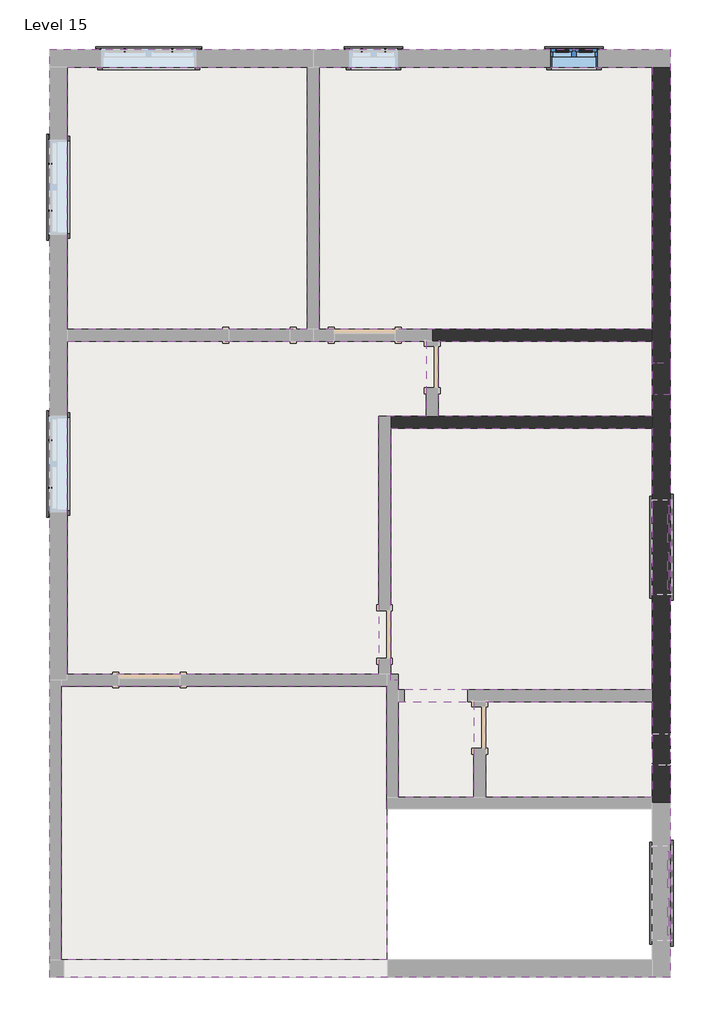
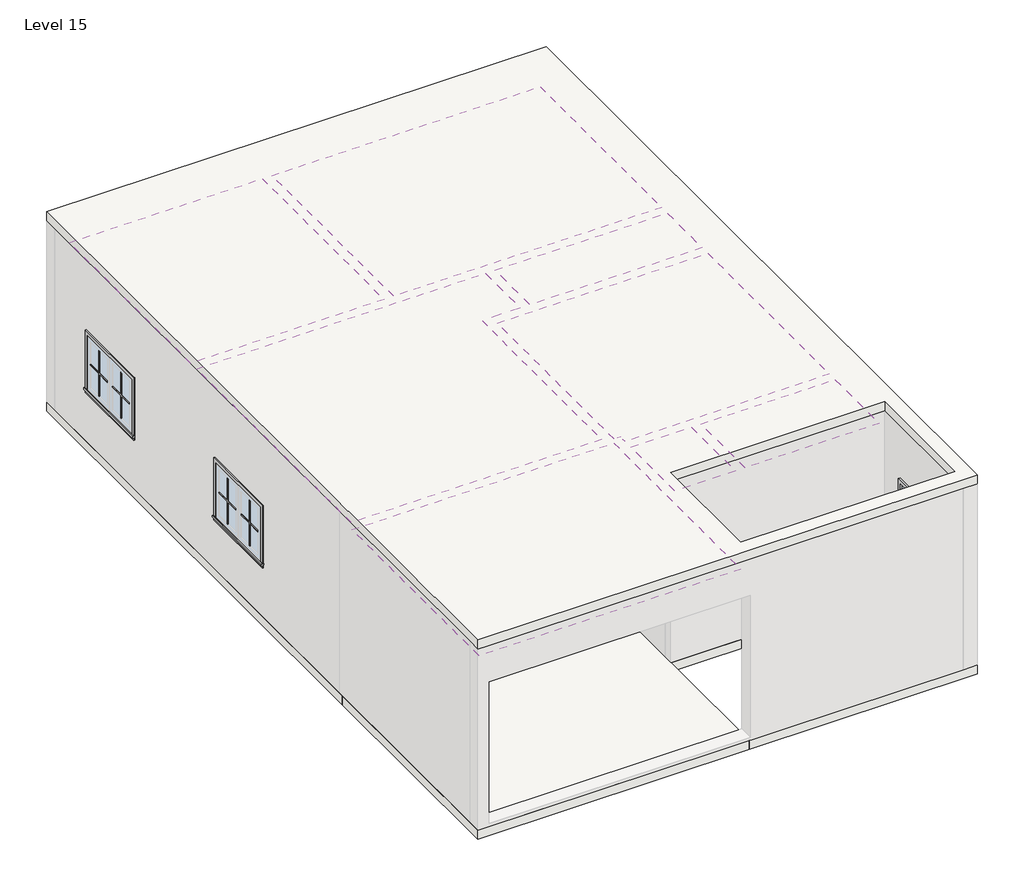
# One storey, part 2 of 2: 44 proxies, 8 coverings, 3 slabs, 3 walls, 3 windows.
"""IFC4 building model written with IfcOpenShell, lengths in millimetres."""

from ifc_helpers import new_model, si_unit, frame, origin, place, context, project, spatial, polyline, outline, extrude, faceted_brep, transform, mapped, element, save
from components import muntin_pattern_2x2_muntin_pattern_2x2_2357e71d, muntin_pattern_2x2_muntin_pattern_2x2_302d8f29, muntin_pattern_2x2_muntin_pattern_2x2_53152e2c, muntin_pattern_2x2_muntin_pattern_2x2_e8f3e573, trim_window_exterior_flat_with_sill_c4e67c73, trim_window_exterior_flat_with_sill_a665a915, trim_window_interior_flat_picture_frame_cf1733af, trim_window_interior_flat_picture_frame_d485c387, fixed_2_415b3208, window_casement_double_3_c417fced

model = new_model("IFC4")

# Units and contexts
model_context = context("Model", 3, world=origin())
ifc_project = project(units=[si_unit("LENGTHUNIT", "METRE", prefix="MILLI")], contexts=[model_context])

# Site, building, storey
site = spatial("IfcSite", under=ifc_project)
building = spatial("IfcBuilding", under=site)
storey = spatial("IfcBuildingStorey", under=building, Name="Level 15", Elevation=6400.8)

# Proxies
placement = place(None, origin())
muntin_pattern_2x2_muntin_pattern_2x2_shape = muntin_pattern_2x2_muntin_pattern_2x2_2357e71d(model_context)
element("IfcBuildingElementProxy", 1, Name="Muntin Pattern_2x2 : Muntin Pattern_2x2", ObjectType="Muntin Pattern_2x2 : Muntin Pattern_2x2", at=placement, inside=storey, context=model_context, shape_type="MappedRepresentation", body=[
    mapped(muntin_pattern_2x2_muntin_pattern_2x2_shape, transform((-4942.3279463, 5897.3080275, 7385.05), x_axis=(1.0, 0.0, 0.0), y_axis=(0.0, 1.0, 0.0), z_axis=(0.0, 0.0, 1.0))),
])
element("IfcBuildingElementProxy", 2, Name="Muntin Pattern_2x2 : Muntin Pattern_2x2", ObjectType="Muntin Pattern_2x2 : Muntin Pattern_2x2", at=placement, inside=storey, context=model_context, shape_type="MappedRepresentation", body=[
    mapped(muntin_pattern_2x2_muntin_pattern_2x2_shape, transform((-5899.5904463, 3838.3205275, 7385.05), x_axis=(0.0, 1.0, 0.0), y_axis=(-1.0, 0.0, 0.0), z_axis=(0.0, 0.0, 1.0))),
])
element("IfcBuildingElementProxy", 3, Name="Muntin Pattern_2x2 : Muntin Pattern_2x2", ObjectType="Muntin Pattern_2x2 : Muntin Pattern_2x2", at=placement, inside=storey, context=model_context, shape_type="MappedRepresentation", body=[
    mapped(muntin_pattern_2x2_muntin_pattern_2x2_shape, transform((-5899.5904463, 293.4330275, 7385.05), x_axis=(0.0, 1.0, 0.0), y_axis=(-1.0, 0.0, 0.0), z_axis=(0.0, 0.0, 1.0))),
])
element("IfcBuildingElementProxy", 4, Name="Muntin Pattern_2x2 : Muntin Pattern_2x2", ObjectType="Muntin Pattern_2x2 : Muntin Pattern_2x2", at=placement, inside=storey, context=model_context, shape_type="MappedRepresentation", body=[
    mapped(muntin_pattern_2x2_muntin_pattern_2x2_shape, transform((2031.5595537, -166.9419725, 7689.85), x_axis=(0.0, -1.0, 0.0), y_axis=(1.0, 0.0, 0.0), z_axis=(0.0, 0.0, 1.0))),
])
element("IfcBuildingElementProxy", 5, Name="Muntin Pattern_2x2 : Muntin Pattern_2x2", ObjectType="Muntin Pattern_2x2 : Muntin Pattern_2x2", at=placement, inside=storey, context=model_context, shape_type="MappedRepresentation", body=[
    mapped(muntin_pattern_2x2_muntin_pattern_2x2_shape, transform((2031.5595537, -4599.2419725, 7689.85), x_axis=(0.0, -1.0, 0.0), y_axis=(1.0, 0.0, 0.0), z_axis=(0.0, 0.0, 1.0))),
])
element("IfcBuildingElementProxy", 6, Name="Muntin Pattern_2x2 : Muntin Pattern_2x2", ObjectType="Muntin Pattern_2x2 : Muntin Pattern_2x2", at=placement, inside=storey, context=model_context, shape_type="MappedRepresentation", body=[
    mapped(muntin_pattern_2x2_muntin_pattern_2x2_shape, transform((-4942.3279463, 5897.3080275, 7385.05), x_axis=(1.0, 0.0, 0.0), y_axis=(0.0, 1.0, 0.0), z_axis=(0.0, 0.0, 1.0))),
])
element("IfcBuildingElementProxy", 7, Name="Muntin Pattern_2x2 : Muntin Pattern_2x2", ObjectType="Muntin Pattern_2x2 : Muntin Pattern_2x2", at=placement, inside=storey, context=model_context, shape_type="MappedRepresentation", body=[
    mapped(muntin_pattern_2x2_muntin_pattern_2x2_shape, transform((2031.5595537, -4599.2419725, 7689.85), x_axis=(0.0, -1.0, 0.0), y_axis=(1.0, 0.0, 0.0), z_axis=(0.0, 0.0, 1.0))),
])
muntin_pattern_2x2_muntin_pattern_2x2_2_shape = muntin_pattern_2x2_muntin_pattern_2x2_302d8f29(model_context)
element("IfcBuildingElementProxy", 8, Name="Muntin Pattern_2x2 : Muntin Pattern_2x2", ObjectType="Muntin Pattern_2x2 : Muntin Pattern_2x2", at=placement, inside=storey, context=model_context, shape_type="MappedRepresentation", body=[
    mapped(muntin_pattern_2x2_muntin_pattern_2x2_2_shape, transform((-4335.9029463, 5897.3080275, 7385.05), x_axis=(-1.0, 0.0, 0.0), y_axis=(0.0, -1.0, 0.0), z_axis=(0.0, 0.0, 1.0))),
])
element("IfcBuildingElementProxy", 9, Name="Muntin Pattern_2x2 : Muntin Pattern_2x2", ObjectType="Muntin Pattern_2x2 : Muntin Pattern_2x2", at=placement, inside=storey, context=model_context, shape_type="MappedRepresentation", body=[
    mapped(muntin_pattern_2x2_muntin_pattern_2x2_2_shape, transform((-5899.5904463, 4444.7455275, 7385.05), x_axis=(0.0, -1.0, 0.0), y_axis=(1.0, 0.0, 0.0), z_axis=(0.0, 0.0, 1.0))),
])
element("IfcBuildingElementProxy", 10, Name="Muntin Pattern_2x2 : Muntin Pattern_2x2", ObjectType="Muntin Pattern_2x2 : Muntin Pattern_2x2", at=placement, inside=storey, context=model_context, shape_type="MappedRepresentation", body=[
    mapped(muntin_pattern_2x2_muntin_pattern_2x2_2_shape, transform((-5899.5904463, 899.8580275, 7385.05), x_axis=(0.0, -1.0, 0.0), y_axis=(1.0, 0.0, 0.0), z_axis=(0.0, 0.0, 1.0))),
])
element("IfcBuildingElementProxy", 11, Name="Muntin Pattern_2x2 : Muntin Pattern_2x2", ObjectType="Muntin Pattern_2x2 : Muntin Pattern_2x2", at=placement, inside=storey, context=model_context, shape_type="MappedRepresentation", body=[
    mapped(muntin_pattern_2x2_muntin_pattern_2x2_2_shape, transform((2031.5595537, -773.3669725, 7689.85), x_axis=(0.0, 1.0, 0.0), y_axis=(-1.0, 0.0, 0.0), z_axis=(0.0, 0.0, 1.0))),
])
element("IfcBuildingElementProxy", 12, Name="Muntin Pattern_2x2 : Muntin Pattern_2x2", ObjectType="Muntin Pattern_2x2 : Muntin Pattern_2x2", at=placement, inside=storey, context=model_context, shape_type="MappedRepresentation", body=[
    mapped(muntin_pattern_2x2_muntin_pattern_2x2_2_shape, transform((2031.5595537, -5205.6669725, 7689.85), x_axis=(0.0, 1.0, 0.0), y_axis=(-1.0, 0.0, 0.0), z_axis=(0.0, 0.0, 1.0))),
])
element("IfcBuildingElementProxy", 13, Name="Muntin Pattern_2x2 : Muntin Pattern_2x2", ObjectType="Muntin Pattern_2x2 : Muntin Pattern_2x2", at=placement, inside=storey, context=model_context, shape_type="MappedRepresentation", body=[
    mapped(muntin_pattern_2x2_muntin_pattern_2x2_2_shape, transform((-4335.9029463, 5897.3080275, 7385.05), x_axis=(-1.0, 0.0, 0.0), y_axis=(0.0, -1.0, 0.0), z_axis=(0.0, 0.0, 1.0))),
])
element("IfcBuildingElementProxy", 14, Name="Muntin Pattern_2x2 : Muntin Pattern_2x2", ObjectType="Muntin Pattern_2x2 : Muntin Pattern_2x2", at=placement, inside=storey, context=model_context, shape_type="MappedRepresentation", body=[
    mapped(muntin_pattern_2x2_muntin_pattern_2x2_2_shape, transform((2031.5595537, -5205.6669725, 7689.85), x_axis=(0.0, 1.0, 0.0), y_axis=(-1.0, 0.0, 0.0), z_axis=(0.0, 0.0, 1.0))),
])
muntin_pattern_2x2_muntin_pattern_2x2_3_shape = muntin_pattern_2x2_muntin_pattern_2x2_53152e2c(model_context)
element("IfcBuildingElementProxy", 15, Name="Muntin Pattern_2x2 : Muntin Pattern_2x2", ObjectType="Muntin Pattern_2x2 : Muntin Pattern_2x2", at=placement, inside=storey, context=model_context, shape_type="MappedRepresentation", body=[
    mapped(muntin_pattern_2x2_muntin_pattern_2x2_3_shape, transform((-1907.0279463, 5897.3080275, 7385.05), x_axis=(1.0, 0.0, 0.0), y_axis=(0.0, 1.0, 0.0), z_axis=(0.0, 0.0, 1.0))),
])
element("IfcBuildingElementProxy", 16, Name="Muntin Pattern_2x2 : Muntin Pattern_2x2", ObjectType="Muntin Pattern_2x2 : Muntin Pattern_2x2", at=placement, inside=storey, context=model_context, shape_type="MappedRepresentation", body=[
    mapped(muntin_pattern_2x2_muntin_pattern_2x2_3_shape, transform((658.3720537, 5897.3080275, 7385.05), x_axis=(1.0, 0.0, 0.0), y_axis=(0.0, 1.0, 0.0), z_axis=(0.0, 0.0, 1.0))),
])
element("IfcBuildingElementProxy", 17, Name="Muntin Pattern_2x2 : Muntin Pattern_2x2", ObjectType="Muntin Pattern_2x2 : Muntin Pattern_2x2", at=placement, inside=storey, context=model_context, shape_type="MappedRepresentation", body=[
    mapped(muntin_pattern_2x2_muntin_pattern_2x2_3_shape, transform((-1907.0279463, 5897.3080275, 7385.05), x_axis=(1.0, 0.0, 0.0), y_axis=(0.0, 1.0, 0.0), z_axis=(0.0, 0.0, 1.0))),
])
element("IfcBuildingElementProxy", 18, Name="Muntin Pattern_2x2 : Muntin Pattern_2x2", ObjectType="Muntin Pattern_2x2 : Muntin Pattern_2x2", at=placement, inside=storey, context=model_context, shape_type="MappedRepresentation", body=[
    mapped(muntin_pattern_2x2_muntin_pattern_2x2_3_shape, transform((658.3720537, 5897.3080275, 7385.05), x_axis=(1.0, 0.0, 0.0), y_axis=(0.0, 1.0, 0.0), z_axis=(0.0, 0.0, 1.0))),
])
muntin_pattern_2x2_muntin_pattern_2x2_4_shape = muntin_pattern_2x2_muntin_pattern_2x2_e8f3e573(model_context)
element("IfcBuildingElementProxy", 19, Name="Muntin Pattern_2x2 : Muntin Pattern_2x2", ObjectType="Muntin Pattern_2x2 : Muntin Pattern_2x2", at=placement, inside=storey, context=model_context, shape_type="MappedRepresentation", body=[
    mapped(muntin_pattern_2x2_muntin_pattern_2x2_4_shape, transform((-1605.4029463, 5897.3080275, 7385.05), x_axis=(-1.0, 0.0, 0.0), y_axis=(0.0, -1.0, 0.0), z_axis=(0.0, 0.0, 1.0))),
])
element("IfcBuildingElementProxy", 20, Name="Muntin Pattern_2x2 : Muntin Pattern_2x2", ObjectType="Muntin Pattern_2x2 : Muntin Pattern_2x2", at=placement, inside=storey, context=model_context, shape_type="MappedRepresentation", body=[
    mapped(muntin_pattern_2x2_muntin_pattern_2x2_4_shape, transform((959.9970537, 5897.3080275, 7385.05), x_axis=(-1.0, 0.0, 0.0), y_axis=(0.0, -1.0, 0.0), z_axis=(0.0, 0.0, 1.0))),
])
element("IfcBuildingElementProxy", 21, Name="Muntin Pattern_2x2 : Muntin Pattern_2x2", ObjectType="Muntin Pattern_2x2 : Muntin Pattern_2x2", at=placement, inside=storey, context=model_context, shape_type="MappedRepresentation", body=[
    mapped(muntin_pattern_2x2_muntin_pattern_2x2_4_shape, transform((-1605.4029463, 5897.3080275, 7385.05), x_axis=(-1.0, 0.0, 0.0), y_axis=(0.0, -1.0, 0.0), z_axis=(0.0, 0.0, 1.0))),
])
element("IfcBuildingElementProxy", 22, Name="Muntin Pattern_2x2 : Muntin Pattern_2x2", ObjectType="Muntin Pattern_2x2 : Muntin Pattern_2x2", at=placement, inside=storey, context=model_context, shape_type="MappedRepresentation", body=[
    mapped(muntin_pattern_2x2_muntin_pattern_2x2_4_shape, transform((959.9970537, 5897.3080275, 7385.05), x_axis=(-1.0, 0.0, 0.0), y_axis=(0.0, -1.0, 0.0), z_axis=(0.0, 0.0, 1.0))),
])
trim_window_exterior_flat_with_sill_shape = trim_window_exterior_flat_with_sill_c4e67c73(model_context)
element("IfcBuildingElementProxy", 23, Name="Trim-Window-Exterior-Flat : with Sill", ObjectType="Trim-Window-Exterior-Flat : with Sill", at=placement, inside=storey, context=model_context, shape_type="MappedRepresentation", body=[
    mapped(trim_window_exterior_flat_with_sill_shape, transform((-4639.1154463, 5906.8330275, 8229.6), x_axis=(-1.0, 0.0, 0.0), y_axis=(0.0, 0.0, 1.0), z_axis=(0.0, 1.0, 0.0))),
])
element("IfcBuildingElementProxy", 24, Name="Trim-Window-Exterior-Flat : with Sill", ObjectType="Trim-Window-Exterior-Flat : with Sill", at=placement, inside=storey, context=model_context, shape_type="MappedRepresentation", body=[
    mapped(trim_window_exterior_flat_with_sill_shape, transform((-5909.1154463, 4141.5330275, 8229.6), x_axis=(0.0, -1.0, 0.0), y_axis=(0.0, 0.0, 1.0), z_axis=(-1.0, 0.0, 0.0))),
])
element("IfcBuildingElementProxy", 25, Name="Trim-Window-Exterior-Flat : with Sill", ObjectType="Trim-Window-Exterior-Flat : with Sill", at=placement, inside=storey, context=model_context, shape_type="MappedRepresentation", body=[
    mapped(trim_window_exterior_flat_with_sill_shape, transform((-5909.1154463, 596.6455275, 8229.6), x_axis=(0.0, -1.0, 0.0), y_axis=(0.0, 0.0, 1.0), z_axis=(-1.0, 0.0, 0.0))),
])
element("IfcBuildingElementProxy", 26, Name="Trim-Window-Exterior-Flat : with Sill", ObjectType="Trim-Window-Exterior-Flat : with Sill", at=placement, inside=storey, context=model_context, shape_type="MappedRepresentation", body=[
    mapped(trim_window_exterior_flat_with_sill_shape, transform((2041.0845537, -470.1544725, 8534.4), x_axis=(0.0, 1.0, 0.0), y_axis=(0.0, 0.0, 1.0), z_axis=(1.0, 0.0, 0.0))),
])
element("IfcBuildingElementProxy", 27, Name="Trim-Window-Exterior-Flat : with Sill", ObjectType="Trim-Window-Exterior-Flat : with Sill", at=placement, inside=storey, context=model_context, shape_type="MappedRepresentation", body=[
    mapped(trim_window_exterior_flat_with_sill_shape, transform((2041.0845537, -4902.4544725, 8534.4), x_axis=(0.0, 1.0, 0.0), y_axis=(0.0, 0.0, 1.0), z_axis=(1.0, 0.0, 0.0))),
])
element("IfcBuildingElementProxy", 28, Name="Trim-Window-Exterior-Flat : with Sill", ObjectType="Trim-Window-Exterior-Flat : with Sill", at=placement, inside=storey, context=model_context, shape_type="MappedRepresentation", body=[
    mapped(trim_window_exterior_flat_with_sill_shape, transform((-4639.1154463, 5906.8330275, 8229.6), x_axis=(-1.0, 0.0, 0.0), y_axis=(0.0, 0.0, 1.0), z_axis=(0.0, 1.0, 0.0))),
])
element("IfcBuildingElementProxy", 29, Name="Trim-Window-Exterior-Flat : with Sill", ObjectType="Trim-Window-Exterior-Flat : with Sill", at=placement, inside=storey, context=model_context, shape_type="MappedRepresentation", body=[
    mapped(trim_window_exterior_flat_with_sill_shape, transform((2041.0845537, -4902.4544725, 8534.4), x_axis=(0.0, 1.0, 0.0), y_axis=(0.0, 0.0, 1.0), z_axis=(1.0, 0.0, 0.0))),
])
trim_window_exterior_flat_with_sill_2_shape = trim_window_exterior_flat_with_sill_a665a915(model_context)
element("IfcBuildingElementProxy", 30, Name="Trim-Window-Exterior-Flat : with Sill", ObjectType="Trim-Window-Exterior-Flat : with Sill", at=placement, inside=storey, context=model_context, shape_type="MappedRepresentation", body=[
    mapped(trim_window_exterior_flat_with_sill_2_shape, transform((-1756.2154463, 5906.8330275, 8229.6), x_axis=(-1.0, 0.0, 0.0), y_axis=(0.0, 0.0, 1.0), z_axis=(0.0, 1.0, 0.0))),
])
element("IfcBuildingElementProxy", 31, Name="Trim-Window-Exterior-Flat : with Sill", ObjectType="Trim-Window-Exterior-Flat : with Sill", at=placement, inside=storey, context=model_context, shape_type="MappedRepresentation", body=[
    mapped(trim_window_exterior_flat_with_sill_2_shape, transform((809.1845537, 5906.8330275, 8229.6), x_axis=(-1.0, 0.0, 0.0), y_axis=(0.0, 0.0, 1.0), z_axis=(0.0, 1.0, 0.0))),
])
element("IfcBuildingElementProxy", 32, Name="Trim-Window-Exterior-Flat : with Sill", ObjectType="Trim-Window-Exterior-Flat : with Sill", at=placement, inside=storey, context=model_context, shape_type="MappedRepresentation", body=[
    mapped(trim_window_exterior_flat_with_sill_2_shape, transform((-1756.2154463, 5906.8330275, 8229.6), x_axis=(-1.0, 0.0, 0.0), y_axis=(0.0, 0.0, 1.0), z_axis=(0.0, 1.0, 0.0))),
])
element("IfcBuildingElementProxy", 33, Name="Trim-Window-Exterior-Flat : with Sill", ObjectType="Trim-Window-Exterior-Flat : with Sill", at=placement, inside=storey, context=model_context, shape_type="MappedRepresentation", body=[
    mapped(trim_window_exterior_flat_with_sill_2_shape, transform((809.1845537, 5906.8330275, 8229.6), x_axis=(-1.0, 0.0, 0.0), y_axis=(0.0, 0.0, 1.0), z_axis=(0.0, 1.0, 0.0))),
])
trim_window_interior_flat_picture_frame_shape = trim_window_interior_flat_picture_frame_cf1733af(model_context)
element("IfcBuildingElementProxy", 34, Name="Trim-Window-Interior-Flat : Picture Frame", ObjectType="Trim-Window-Interior-Flat : Picture Frame", at=placement, inside=storey, context=model_context, shape_type="MappedRepresentation", body=[
    mapped(trim_window_interior_flat_picture_frame_shape, transform((-4639.1154463, 5678.2330275, 8229.6), x_axis=(1.0, 0.0, 0.0), y_axis=(0.0, 0.0, 1.0), z_axis=(0.0, -1.0, 0.0))),
])
element("IfcBuildingElementProxy", 35, Name="Trim-Window-Interior-Flat : Picture Frame", ObjectType="Trim-Window-Interior-Flat : Picture Frame", at=placement, inside=storey, context=model_context, shape_type="MappedRepresentation", body=[
    mapped(trim_window_interior_flat_picture_frame_shape, transform((-5680.5154463, 4141.5330275, 8229.6), x_axis=(0.0, 1.0, 0.0), y_axis=(0.0, 0.0, 1.0), z_axis=(1.0, 0.0, 0.0))),
])
element("IfcBuildingElementProxy", 36, Name="Trim-Window-Interior-Flat : Picture Frame", ObjectType="Trim-Window-Interior-Flat : Picture Frame", at=placement, inside=storey, context=model_context, shape_type="MappedRepresentation", body=[
    mapped(trim_window_interior_flat_picture_frame_shape, transform((-5680.5154463, 596.6455275, 8229.6), x_axis=(0.0, 1.0, 0.0), y_axis=(0.0, 0.0, 1.0), z_axis=(1.0, 0.0, 0.0))),
])
element("IfcBuildingElementProxy", 37, Name="Trim-Window-Interior-Flat : Picture Frame", ObjectType="Trim-Window-Interior-Flat : Picture Frame", at=placement, inside=storey, context=model_context, shape_type="MappedRepresentation", body=[
    mapped(trim_window_interior_flat_picture_frame_shape, transform((1812.4845537, -470.1544725, 8534.4), x_axis=(0.0, -1.0, 0.0), y_axis=(0.0, 0.0, 1.0), z_axis=(-1.0, 0.0, 0.0))),
])
element("IfcBuildingElementProxy", 38, Name="Trim-Window-Interior-Flat : Picture Frame", ObjectType="Trim-Window-Interior-Flat : Picture Frame", at=placement, inside=storey, context=model_context, shape_type="MappedRepresentation", body=[
    mapped(trim_window_interior_flat_picture_frame_shape, transform((1812.4845537, -4902.4544725, 8534.4), x_axis=(0.0, -1.0, 0.0), y_axis=(0.0, 0.0, 1.0), z_axis=(-1.0, 0.0, 0.0))),
])
element("IfcBuildingElementProxy", 39, Name="Trim-Window-Interior-Flat : Picture Frame", ObjectType="Trim-Window-Interior-Flat : Picture Frame", at=placement, inside=storey, context=model_context, shape_type="MappedRepresentation", body=[
    mapped(trim_window_interior_flat_picture_frame_shape, transform((-4639.1154463, 5678.2330275, 8229.6), x_axis=(1.0, 0.0, 0.0), y_axis=(0.0, 0.0, 1.0), z_axis=(0.0, -1.0, 0.0))),
])
element("IfcBuildingElementProxy", 40, Name="Trim-Window-Interior-Flat : Picture Frame", ObjectType="Trim-Window-Interior-Flat : Picture Frame", at=placement, inside=storey, context=model_context, shape_type="MappedRepresentation", body=[
    mapped(trim_window_interior_flat_picture_frame_shape, transform((1812.4845537, -4902.4544725, 8534.4), x_axis=(0.0, -1.0, 0.0), y_axis=(0.0, 0.0, 1.0), z_axis=(-1.0, 0.0, 0.0))),
])
trim_window_interior_flat_picture_frame_2_shape = trim_window_interior_flat_picture_frame_d485c387(model_context)
element("IfcBuildingElementProxy", 41, Name="Trim-Window-Interior-Flat : Picture Frame", ObjectType="Trim-Window-Interior-Flat : Picture Frame", at=placement, inside=storey, context=model_context, shape_type="MappedRepresentation", body=[
    mapped(trim_window_interior_flat_picture_frame_2_shape, transform((-1756.2154463, 5678.2330275, 8229.6), x_axis=(1.0, 0.0, 0.0), y_axis=(0.0, 0.0, 1.0), z_axis=(0.0, -1.0, 0.0))),
])
element("IfcBuildingElementProxy", 42, Name="Trim-Window-Interior-Flat : Picture Frame", ObjectType="Trim-Window-Interior-Flat : Picture Frame", at=placement, inside=storey, context=model_context, shape_type="MappedRepresentation", body=[
    mapped(trim_window_interior_flat_picture_frame_2_shape, transform((809.1845537, 5678.2330275, 8229.6), x_axis=(1.0, 0.0, 0.0), y_axis=(0.0, 0.0, 1.0), z_axis=(0.0, -1.0, 0.0))),
])
element("IfcBuildingElementProxy", 43, Name="Trim-Window-Interior-Flat : Picture Frame", ObjectType="Trim-Window-Interior-Flat : Picture Frame", at=placement, inside=storey, context=model_context, shape_type="MappedRepresentation", body=[
    mapped(trim_window_interior_flat_picture_frame_2_shape, transform((-1756.2154463, 5678.2330275, 8229.6), x_axis=(1.0, 0.0, 0.0), y_axis=(0.0, 0.0, 1.0), z_axis=(0.0, -1.0, 0.0))),
])
element("IfcBuildingElementProxy", 44, Name="Trim-Window-Interior-Flat : Picture Frame", ObjectType="Trim-Window-Interior-Flat : Picture Frame", at=placement, inside=storey, context=model_context, shape_type="MappedRepresentation", body=[
    mapped(trim_window_interior_flat_picture_frame_2_shape, transform((809.1845537, 5678.2330275, 8229.6), x_axis=(1.0, 0.0, 0.0), y_axis=(0.0, 0.0, 1.0), z_axis=(0.0, -1.0, 0.0))),
])

# Coverings
element("IfcCovering", 45, ObjectType="2' x 4' ACT System", at=placement, inside=storey, context=model_context, shape_type="SweptSolid", body=[
    extrude(outline(polyline([(-5680.5154463, 2323.8455275), (-5680.5154463, 5678.2330275), (-2607.1154463, 5678.2330275), (-2607.1154463, 2323.8455275), (-5680.5154463, 2323.8455275)])), frame((0.0, 0.0, 9144.0), z_axis=(0.0, 0.0, 1.0), x_axis=(1.0, 0.0, 0.0)), (0.0, 0.0, 1.0), 57.15),
])
element("IfcCovering", 46, ObjectType="2' x 4' ACT System", at=placement, inside=storey, context=model_context, shape_type="SweptSolid", body=[
    extrude(outline(polyline([(-2454.7154463, 2323.8455275), (-2454.7154463, 5678.2330275), (1812.4845537, 5678.2330275), (1812.4845537, 2323.8455275), (-2454.7154463, 2323.8455275)])), frame((0.0, 0.0, 9144.0), z_axis=(0.0, 0.0, 1.0), x_axis=(1.0, 0.0, 0.0)), (0.0, 0.0, 1.0), 57.15),
])
element("IfcCovering", 47, ObjectType="2' x 4' ACT System", at=placement, inside=storey, context=model_context, shape_type="SweptSolid", body=[
    extrude(outline(polyline([(-5680.5154463, -2095.7544725), (-5680.5154463, 2171.4455275), (-1083.1154463, 2171.4455275), (-1083.1154463, 1206.2455275), (-1692.7154463, 1206.2455275), (-1692.7154463, -2095.7544725), (-5680.5154463, -2095.7544725)])), frame((0.0, 0.0, 9144.0), z_axis=(0.0, 0.0, 1.0), x_axis=(1.0, 0.0, 0.0)), (0.0, 0.0, 1.0), 57.15),
])
element("IfcCovering", 48, ObjectType="2' x 4' ACT System", at=placement, inside=storey, context=model_context, shape_type="SweptSolid", body=[
    extrude(outline(polyline([(-930.7154463, 2171.4455275), (1812.4845537, 2171.4455275), (1812.4845537, 1206.2455275), (-930.7154463, 1206.2455275), (-930.7154463, 2171.4455275)])), frame((0.0, 0.0, 9144.0), z_axis=(0.0, 0.0, 1.0), x_axis=(1.0, 0.0, 0.0)), (0.0, 0.0, 1.0), 57.15),
])
element("IfcCovering", 49, ObjectType="2' x 4' ACT System", at=placement, inside=storey, context=model_context, shape_type="SweptSolid", body=[
    extrude(outline(polyline([(1812.4845537, 1053.8455275), (1812.4845537, -2298.9544725), (-1438.7154463, -2298.9544725), (-1438.7154463, -2171.9544725), (-1540.3154463, -2171.9544725), (-1540.3154463, 1053.8455275), (1812.4845537, 1053.8455275)])), frame((0.0, 0.0, 9144.0), z_axis=(0.0, 0.0, 1.0), x_axis=(1.0, 0.0, 0.0)), (0.0, 0.0, 1.0), 57.15),
])
element("IfcCovering", 50, ObjectType="2' x 4' ACT System", at=placement, inside=storey, context=model_context, shape_type="SweptSolid", body=[
    extrude(outline(polyline([(1812.4845537, -2451.3544725), (1812.4845537, -3670.5544725), (-321.1154463, -3670.5544725), (-321.1154463, -2451.3544725), (1812.4845537, -2451.3544725)])), frame((0.0, 0.0, 9144.0), z_axis=(0.0, 0.0, 1.0), x_axis=(1.0, 0.0, 0.0)), (0.0, 0.0, 1.0), 57.15),
])
element("IfcCovering", 51, ObjectType="2' x 4' ACT System", at=placement, inside=storey, context=model_context, shape_type="SweptSolid", body=[
    extrude(outline(polyline([(-473.5154463, -2451.3544725), (-473.5154463, -3670.5544725), (-1438.7154463, -3670.5544725), (-1438.7154463, -2451.3544725), (-473.5154463, -2451.3544725)])), frame((0.0, 0.0, 9144.0), z_axis=(0.0, 0.0, 1.0), x_axis=(1.0, 0.0, 0.0)), (0.0, 0.0, 1.0), 57.15),
])
element("IfcCovering", 52, ObjectType="2' x 4' ACT System", at=placement, inside=storey, context=model_context, shape_type="SweptSolid", body=[
    extrude(outline(polyline([(-1591.1154463, -2248.1544725), (-1591.1154463, -5753.3544725), (-5756.7154463, -5753.3544725), (-5756.7154463, -2248.1544725), (-1591.1154463, -2248.1544725)])), frame((0.0, 0.0, 9144.0), z_axis=(0.0, 0.0, 1.0), x_axis=(1.0, 0.0, 0.0)), (0.0, 0.0, 1.0), 57.15),
])

# Slabs
element("IfcSlab", 53, ObjectType="Generic - 6\"", at=placement, inside=storey, context=model_context, shape_type="SweptSolid", body=[
    extrude(outline(polyline([(-5909.1154463, -2248.1544725), (-5909.1154463, 5906.8330275), (2041.0845537, 5906.8330275), (2041.0845537, -5981.9544725), (-1591.1154463, -5981.9544725), (-1591.1154463, -5753.3544725), (1812.4845537, -5753.3544725), (1812.4845537, -3822.9544725), (-1591.1154463, -3822.9544725), (-1591.1154463, -2248.1544725), (-5756.7154463, -2248.1544725), (-5909.1154463, -2248.1544725)])), frame((0.0, 0.0, 6248.4), z_axis=(0.0, 0.0, 1.0), x_axis=(1.0, 0.0, 0.0)), (0.0, 0.0, 1.0), 152.4),
])
element("IfcSlab", 54, ObjectType="Generic - 6\"", at=placement, inside=storey, context=model_context, shape_type="SweptSolid", body=[
    extrude(outline(polyline([(-1591.1154463, -2248.1544725), (-1591.1154463, -5981.9544725), (-5909.1154463, -5981.9544725), (-5909.1154463, -2248.1544725), (-1591.1154463, -2248.1544725)])), frame((0.0, 0.0, 6248.4), z_axis=(0.0, 0.0, 1.0), x_axis=(1.0, 0.0, 0.0)), (0.0, 0.0, 1.0), 152.4),
])
element("IfcSlab", 55, ObjectType="Generic - 6\"", at=placement, inside=storey, context=model_context, shape_type="SweptSolid", body=[
    extrude(outline(polyline([(2041.0845537, 5906.8330275), (2041.0845537, -5981.9544725), (-5909.1154463, -5981.9544725), (-5909.1154463, 5906.8330275), (2041.0845537, 5906.8330275)]), holes=[polyline([(1812.4845537, -3822.9544725), (-1591.1154463, -3822.9544725), (-1591.1154463, -5753.3544725), (1812.4845537, -5753.3544725), (1812.4845537, -3822.9544725)])]), frame((0.0, 0.0, 9448.8), z_axis=(0.0, 0.0, 1.0), x_axis=(1.0, 0.0, 0.0)), (0.0, 0.0, 1.0), 152.4),
])

# Walls
element("IfcWall", 56, ObjectType="Generic - 6\"", at=placement, inside=storey, context=model_context, shape_type="Brep", body=[
    faceted_brep([(-1540.3154463, 1053.8455275, 6400.8), (1812.4845537, 1053.8455275, 6400.8), (1812.4845537, 1053.8455275, 9448.8), (-1540.3154463, 1053.8455275, 9448.8), (-1540.3154463, 1206.2455275, 6400.8), (-1540.3154463, 1206.2455275, 9448.8), (-1083.1154463, 1206.2455275, 9448.8), (-930.7154463, 1206.2455275, 9448.8), (1812.4845537, 1206.2455275, 9448.8), (1812.4845537, 1206.2455275, 6400.8), (-930.7154463, 1206.2455275, 6400.8), (-1083.1154463, 1206.2455275, 6400.8)], [[[0, 1, 2, 3]], [[4, 5, 6, 7, 8, 9, 10, 11]], [[1, 0, 4, 11, 10, 9]], [[3, 2, 8, 7, 6, 5]], [[0, 3, 5, 4]], [[2, 1, 9, 8]]]),
])
element("IfcWall", 57, ObjectType="Generic - 6\"", at=placement, inside=storey, context=model_context, shape_type="Brep", body=[
    faceted_brep([(1812.4845537, 2323.8455275, 6400.8), (-1006.9154463, 2323.8455275, 6400.8), (-1006.9154463, 2323.8455275, 9448.8), (1812.4845537, 2323.8455275, 9448.8), (1812.4845537, 2171.4455275, 6400.8), (1812.4845537, 2171.4455275, 9448.8), (-930.7154463, 2171.4455275, 9448.8), (-1006.9154463, 2171.4455275, 9448.8), (-1006.9154463, 2171.4455275, 6400.8), (-930.7154463, 2171.4455275, 6400.8)], [[[0, 1, 2, 3]], [[4, 5, 6, 7, 8, 9]], [[1, 0, 4, 9, 8]], [[2, 1, 8, 7]], [[3, 2, 7, 6, 5]], [[0, 3, 5, 4]]]),
])
element("IfcWall", 58, ObjectType="Generic - 9\"", at=placement, inside=storey, context=model_context, shape_type="Brep", body=[
    faceted_brep([(1812.4845537, 5678.2330275, 6400.8), (1812.4845537, 2323.8455275, 6400.8), (1812.4845537, 2171.4455275, 6400.8), (1812.4845537, 1206.2455275, 6400.8), (1812.4845537, 1053.8455275, 6400.8), (1812.4845537, -2298.9544725, 6400.8), (1812.4845537, -2451.3544725, 6400.8), (1812.4845537, -3670.5544725, 6400.8), (1812.4845537, -3746.7544725, 6400.8), (1812.4845537, -3746.7544725, 9448.8), (1812.4845537, -3670.5544725, 9448.8), (1812.4845537, -2451.3544725, 9448.8), (1812.4845537, -2298.9544725, 9448.8), (1812.4845537, 1053.8455275, 9448.8), (1812.4845537, 1206.2455275, 9448.8), (1812.4845537, 2171.4455275, 9448.8), (1812.4845537, 2323.8455275, 9448.8), (1812.4845537, 5678.2330275, 9448.8), (1812.4845537, -1079.7544725, 8534.4), (1812.4845537, -1079.7544725, 7620.0), (1812.4845537, 139.4455275, 7620.0), (1812.4845537, 139.4455275, 8534.4), (1812.4845537, -3264.1544725, 8839.2), (1812.4845537, -3264.1544725, 8229.6), (1812.4845537, -2857.7544725, 8229.6), (1812.4845537, -2857.7544725, 8839.2), (1812.4845537, 1892.0455275, 8839.2), (1812.4845537, 1485.6455275, 8839.2), (1812.4845537, 1485.6455275, 8229.6), (1812.4845537, 1892.0455275, 8229.6), (2041.0845537, 5678.2330275, 6400.8), (2041.0845537, 5678.2330275, 9448.8), (2041.0845537, -3746.7544725, 9448.8), (2041.0845537, -3746.7544725, 6400.8), (2041.0845537, -1079.7544725, 8534.4), (2041.0845537, 139.4455275, 8534.4), (2041.0845537, 139.4455275, 7620.0), (2041.0845537, -1079.7544725, 7620.0), (2041.0845537, -3264.1544725, 8839.2), (2041.0845537, -2857.7544725, 8839.2), (2041.0845537, -2857.7544725, 8229.6), (2041.0845537, -3264.1544725, 8229.6), (2041.0845537, 1892.0455275, 8839.2), (2041.0845537, 1892.0455275, 8229.6), (2041.0845537, 1485.6455275, 8229.6), (2041.0845537, 1485.6455275, 8839.2)], [[[0, 1, 2, 3, 4, 5, 6, 7, 8, 9, 10, 11, 12, 13, 14, 15, 16, 17], [18, 19, 20, 21], [22, 23, 24, 25], [26, 27, 28, 29]], [[30, 31, 32, 33], [34, 35, 36, 37], [38, 39, 40, 41], [42, 43, 44, 45]], [[8, 7, 6, 5, 4, 3, 2, 1, 0, 30, 33]], [[9, 8, 33, 32]], [[17, 16, 15, 14, 13, 12, 11, 10, 9, 32, 31]], [[0, 17, 31, 30]], [[19, 18, 34, 37]], [[20, 19, 37, 36]], [[21, 20, 36, 35]], [[18, 21, 35, 34]], [[23, 22, 38, 41]], [[24, 23, 41, 40]], [[25, 24, 40, 39]], [[22, 25, 39, 38]], [[43, 42, 26, 29]], [[44, 43, 29, 28]], [[45, 44, 28, 27]], [[42, 45, 27, 26]]]),
])

# Windows
fixed_2_shape = fixed_2_415b3208(model_context)
element("IfcWindow", 59, ObjectType="Fixed : 2'", at=placement, inside=storey, context=model_context, shape_type="MappedRepresentation", body=[
    mapped(fixed_2_shape, transform((1926.7845537, 1726.9455275, 7924.8), x_axis=(0.0, 1.0, 0.0), y_axis=(-1.0, 0.0, 0.0), z_axis=(0.0, 0.0, 1.0))),
])
window_casement_double_3_shape = window_casement_double_3_c417fced(model_context)
element("IfcWindow", 60, ObjectType="Window-Casement-Double : 3'", at=placement, inside=storey, context=model_context, shape_type="MappedRepresentation", body=[
    mapped(window_casement_double_3_shape, transform((809.1845537, 5792.5330275, 6400.8), x_axis=(1.0, 0.0, 0.0), y_axis=(0.0, 1.0, 0.0), z_axis=(0.0, 0.0, 1.0))),
])
element("IfcWindow", 61, ObjectType="Window-Casement-Double : 3'", at=placement, inside=storey, context=model_context, shape_type="MappedRepresentation", body=[
    mapped(window_casement_double_3_shape, transform((809.1845537, 5792.5330275, 6400.8), x_axis=(1.0, 0.0, 0.0), y_axis=(0.0, 1.0, 0.0), z_axis=(0.0, 0.0, 1.0))),
])

save(model, "model.ifc")

# Revit data of these elements
# Type "Muntin Pattern_2x2 : Muntin Pattern_2x2"
#   Width [instance default] = 4' - 0"
#   Thickness = 0' - 0 1/2"
#   Height [instance default] = 4' - 0"
#   Distance = 0' - 0 3/4"
#   Interior Material [instance default] = none
#   Exterior Material [instance default] = none
#   Default Elevation = 0
# Type "Trim-Window-Exterior-Flat : with Sill"
#   Trim Width = 0' - 2 1/4"
#   Trim Thickness_Picture Frame = 0' - 1 1/4"
#   Trim Thickness_with Sill = 0' - 0 3/4"
#   Sill Thickness = 0' - 1 1/4"
#   Opening Width [instance default] = 2' - 0"
#   Opening Height [instance default] = 3' - 0"
#   Default Elevation = 4' - 0"
#   Sill = yes
#   Picture Frame = no
#   Trim Material [instance default] = none
# Type "Trim-Window-Interior-Flat : Picture Frame"
#   Trim Thickness_Picture Frame = 0' - 1 1/4"
#   Trim Width = 0' - 2 1/4"
#   Trim Thickness_with Sill = 0' - 0 3/4"
#   Sill Thickness = 0' - 1 1/4"
#   Opening Width [instance default] = 2' - 0"
#   Opening Height [instance default] = 3' - 0"
#   Default Elevation = 4' - 0"
#   Sill = no
#   Picture Frame = yes
#   Trim Material [instance default] = none
# Type "2' x 4' ACT System"
#   Assembly Code = "C3030210"
#   built-in parameter 1002203 = 1 (stored number, unit not read)
#   built-in parameter 1002202 = 1 (stored number, unit not read)
#   Layers, outside or top first: 0' - 1 5/8" "Default" (function 1); 0' - 0 5/8" "Acoustic Ceiling Tile 24 x 48" (function 5)
# Type "Generic - 6\""
#   Assembly Code = "B1010"
#   Function = 0
#   Layers, outside or top first: 0' - 6" no material (function 1)
# Type "Generic - 6\""
#   Assembly Code = "B2010"
#   Layers, outside or top first: 0' - 6" no material (function 1)
# Type "Generic - 9\""
#   Assembly Code = "B2010"
#   Layers, outside or top first: 0' - 9" no material (function 1)
# Type "Fixed : 2'"
#   Type Mark = "20"
#   Construction Type Id = "GSP4R"
#   Assembly Code = "B2020100"
#   Analytic Construction = "1/8 in Pilkington single glazing"
#   Visual Light Transmittance = 0.9
#   Solar Heat Gain Coefficient = 0.78
#   Heat Transfer Coefficient (U) = 0.6496 BTU/(h·ft²·°F)
#   Height = 2' - 0"
#   Default Sill Height = 1' - 0"
#   Width = 1' - 4"
#   Window Inset = 0' - 0 3/4"
#   Define Thermal Properties by = 1
#   Glass Pane Material = Glass
#   Sash Material = Sash
#   Wall Closure = (empty or 0)
# Type "Window-Casement-Double : 3'"
#   Type Mark = "19"
#   Fire Rating = "0.5h"
#   Assembly Code = "B2020100"
#   Analytic Construction = "Double glazing - domestic"
#   Frame Extension [instance default] = 0' - 0 1/4"
#   Window Inset [instance default] = 0' - 0"
#   Wall Thickness [instance default] = 0' - 6"
#   Interior Wall Closure [instance default] = 0' - 2 1/4"
#   Half Width = 1' - 0"
#   Visual Light Transmittance = 0.81
#   Thermal Resistance (R) = 1.8146 (h·ft²·°F)/BTU
#   Solar Heat Gain Coefficient = 0.76
#   Rough Width = 2' - 0 1/2"
#   Rough Height = 3' - 0 1/2"
#   Height = 3' - 0"
#   Heat Transfer Coefficient (U) = 0.5511 BTU/(h·ft²·°F)
#   Exterior Wall Closure [instance default] = 0' - 1 1/4"
#   Extension Jamb [instance default] = 0' - 2 1/4"
#   Default Sill Height = 3' - 0"
#   Width = 2' - 0"
#   Muntin Visibility = yes
#   Interior Trim Visibility [instance default] = yes
#   Exterior Trim Visibility [instance default] = yes
#   Extension Jamb Visibility [instance default] = yes
#   Interior Trim Material = Wood - Stained
#   Muntin Pattern = Muntin Pattern_2x2 : Muntin Pattern_2x2
#   Interior Trim = Trim-Window-Interior-Flat : Picture Frame
#   Interior Frame Material = Wood - Stained
#   Glass Panel Material = Glass
#   Exterior Trim Material = Clad - White
#   Exterior Trim = Trim-Window-Exterior-Flat : with Sill
#   Exterior Frame Material = Clad - White
#   Wall Closure = (empty or 0)
# Elements 1, 2, 3, 4, 5, 6, 7, 8, 9, 10, 11, 12, 13, 14 (IfcBuildingElementProxy, "Muntin Pattern_2x2 : Muntin Pattern_2x2")
#   Width = 1' - 6 5/8"
#   Height = 2' - 6 1/2"
#   Interior Material = Wood - Stained
#   Exterior Material = Clad - White
#   Phase Created = New Construction
#   Materials on its faces: "Clad - White", "Wood - Stained"
# Elements 15, 16, 17, 18, 19, 20, 21, 22 (IfcBuildingElementProxy, "Muntin Pattern_2x2 : Muntin Pattern_2x2")
#   Width = 0' - 6 5/8"
#   Height = 2' - 6 1/2"
#   Interior Material = Wood - Stained
#   Exterior Material = Clad - White
#   Phase Created = New Construction
#   Materials on its faces: "Clad - White", "Wood - Stained"
# Elements 23, 24, 25, 26, 27, 28, 29 (IfcBuildingElementProxy, "Trim-Window-Exterior-Flat : with Sill")
#   Opening Width = 4' - 0"
#   Opening Height = 3' - 0"
#   Trim Material = Clad - White
#   Phase Created = New Construction
#   Materials on its faces: "Clad - White"
# Elements 30, 31, 32, 33 (IfcBuildingElementProxy, "Trim-Window-Exterior-Flat : with Sill")
#   Opening Width = 2' - 0"
#   Opening Height = 3' - 0"
#   Trim Material = Clad - White
#   Phase Created = New Construction
#   Materials on its faces: "Clad - White"
# Elements 34, 35, 36, 37, 38, 39, 40 (IfcBuildingElementProxy, "Trim-Window-Interior-Flat : Picture Frame")
#   Opening Width = 4' - 0"
#   Opening Height = 3' - 0"
#   Trim Material = Wood - Stained
#   Phase Created = New Construction
#   Materials on its faces: "Wood - Stained"
# Elements 41, 42, 43, 44 (IfcBuildingElementProxy, "Trim-Window-Interior-Flat : Picture Frame")
#   Opening Width = 2' - 0"
#   Opening Height = 3' - 0"
#   Trim Material = Wood - Stained
#   Phase Created = New Construction
#   Materials on its faces: "Wood - Stained"
# Elements 45, 46, 47, 48, 49, 50, 51, 52 (IfcCovering, "2' x 4' ACT System")
#   Height Offset From Level = 9' - 0"
#   Phase Created = New Construction
#   Materials on its faces: "Acoustic Ceiling Tile 24 x 48", "Default"
# Element 53 (IfcSlab, "Generic - 6\"")
#   built-in parameter 1001955 = -1.5708 (stored number, unit not read)
#   Height Offset From Level = 0' - 0"
#   Phase Created = New Construction
#   Materials on its faces: "Default Floor", "TILE"
# Element 54 (IfcSlab, "Generic - 6\"")
#   Height Offset From Level = 0' - 0"
#   Phase Created = New Construction
#   Materials on its faces: "Default Floor", "Grass"
# Element 55 (IfcSlab, "Generic - 6\"")
#   Height Offset From Level = 10' - 6"
#   Phase Created = New Construction
#   Materials on its faces: "Default Floor"
# Element 56 (IfcWall, "Generic - 6\"")
#   Top Offset = 0' - 0"
#   Base Offset = 0' - 0"
#   Unconnected Height = 10' - 0"
#   wall height = 10' - 0"
#   Phase Created = New Construction
#   Base Constraint = Level 15
#   Materials on its faces: "Default Wall", "WALL PAINT 4", "WALL PAINT 5"
# Element 57 (IfcWall, "Generic - 6\"")
#   Top Offset = 0' - 0"
#   Base Offset = 0' - 0"
#   Unconnected Height = 10' - 0"
#   wall height = 10' - 0"
#   Phase Created = New Construction
#   Base Constraint = Level 15
#   Materials on its faces: "Default Wall", "WALL PAINT 3", "WALL PAINT 5"
# Element 58 (IfcWall, "Generic - 9\"")
#   Top Offset = 0' - 0"
#   Base Offset = 0' - 0"
#   Unconnected Height = 10' - 0"
#   wall height = 10' - 0"
#   Phase Created = New Construction
#   Base Constraint = Level 15
#   Materials on its faces: "Default Wall"
# Element 59 (IfcWindow, "Fixed : 2'")
#   Mark = "48"
#   Phase Created = New Construction
#   Materials on its faces: "Sash", "Glass"
# Element 60 (IfcWindow, "Window-Casement-Double : 3'")
#   Mark = "46"
#   Window Inset = 0' - 0"
#   Interior Wall Closure = 0' - 2 1/4"
#   Frame Extension = 0' - 0 1/4"
#   Exterior Wall Closure = 0' - 1 1/4"
#   Interior Trim Visibility = yes
#   Exterior Trim Visibility = yes
#   Phase Created = New Construction
#   Materials on its faces: "Wood - Stained", "Glass", "Clad - White"
# Element 61 (IfcWindow, "Window-Casement-Double : 3'")
#   Mark = "52"
#   Window Inset = 0' - 0"
#   Interior Wall Closure = 0' - 2 1/4"
#   Frame Extension = 0' - 0 1/4"
#   Exterior Wall Closure = 0' - 1 1/4"
#   Interior Trim Visibility = yes
#   Exterior Trim Visibility = yes
#   Phase Created = New Construction
#   Materials on its faces: "Wood - Stained", "Glass", "Clad - White"
# Materials
#   "Default": colour RGB 127 127 127, transparency 0, Cost = 0
#   "Acoustic Ceiling Tile 24 x 48": class "Generic", colour RGB 229 229 229, transparency 0, Description = "Acoustic Ceiling Tile 24 x 48", Cost = 0
#   "Glass": class "Glass", colour RGB 0 128 192, transparency 0.75, Description = "Soda Lime Glass", Cost = 0
#   "Sash": class "Wood", colour RGB 224 178 126, transparency 0, Cost = 0
#   "Wood - Stained": class "Wood", colour RGB 224 178 126, transparency 0, Cost = 0
#   "Clad - White": class "Wood", colour RGB 242 242 238, transparency 0, Cost = 0
#   "Default Floor": colour RGB 128 128 128, transparency 0, Cost = 0
#   "TILE": class "Generic", colour RGB 120 120 120, transparency 0, Cost = 0
#   "Grass": class "Generic", colour RGB 104 137 66, transparency 0, Description = "Physical material.", Cost = 0
#   "Default Wall": colour RGB 128 128 128, transparency 0, Cost = 0
#   "WALL PAINT 4": class "Generic", colour RGB 120 120 120, transparency 0, Cost = 0
#   "WALL PAINT 5": class "Generic", colour RGB 120 120 120, transparency 0, Cost = 0
#   "WALL PAINT 3": class "Generic", colour RGB 120 120 120, transparency 0, Cost = 0
